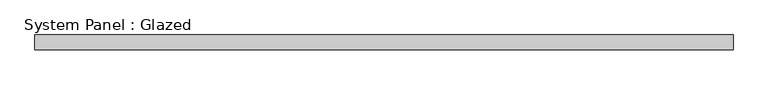
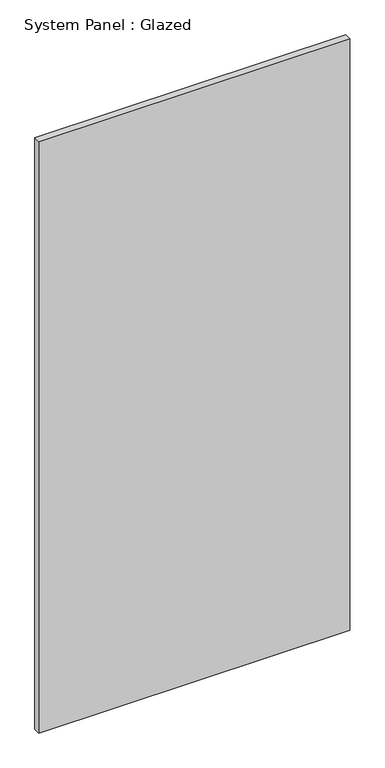
"""IFC4 building model written with IfcOpenShell, lengths in millimetres: plate geometry, System Panel : Glazed."""

from ifc_helpers import new_model, si_unit, origin, origin_with_axes, place, context, project, spatial, polyline, outline, extrude, source, transform, mapped, element, save


def system_panel_glazed_ad55aef1(model_context):
    return source(origin(), model_context, "Body", "SweptSolid", [
        extrude(outline(polyline([(596.6666667, -49.5), (-596.6666667, -49.5), (-596.6666667, -24.5), (596.6666667, -24.5), (596.6666667, -49.5)])), origin_with_axes(), (0.0, 0.0, 1.0), 2400.0),
    ])


if __name__ == "__main__":
    model = new_model("IFC4")
    model_context = context("Model", 3, world=origin())
    ifc_project = project(units=[si_unit("LENGTHUNIT", "METRE", prefix="MILLI")], contexts=[model_context])
    site = spatial("IfcSite", under=ifc_project)
    building = spatial("IfcBuilding", under=site)
    placement = place(None, origin())
    system_panel_glazed_shape = system_panel_glazed_ad55aef1(model_context)
    element("IfcPlate", 1, ObjectType="System Panel : Glazed", at=placement, inside=building, context=model_context, shape_type="MappedRepresentation", body=[
        mapped(system_panel_glazed_shape, transform((0.0, 0.0, 0.0), x_axis=(1.0, 0.0, 0.0), y_axis=(0.0, 1.0, 0.0), z_axis=(0.0, 0.0, 1.0))),
    ])
    save(model, "model.ifc")

# Revit data of these elements
# Type "System Panel : Glazed"
#   Keynote = "H11"
#   Construction Type Id = "GSP4R"
#   Analytic Construction = "1/8 in Pilkington single glazing"
#   Visual Light Transmittance = 0.9
#   Solar Heat Gain Coefficient = 0.86
#   Heat Transfer Coefficient (U) = 6.7069 W/(m²·K)
#   Define Thermal Properties by = 1
# Element 1 (IfcPlate, "System Panel : Glazed")
#   Materials on its faces: "Glass"
# Materials
#   "Glass": class "Glass", colour RGB 0 128 192, transparency 0.9, Description = "Soda Lime Glass", Cost = 0
